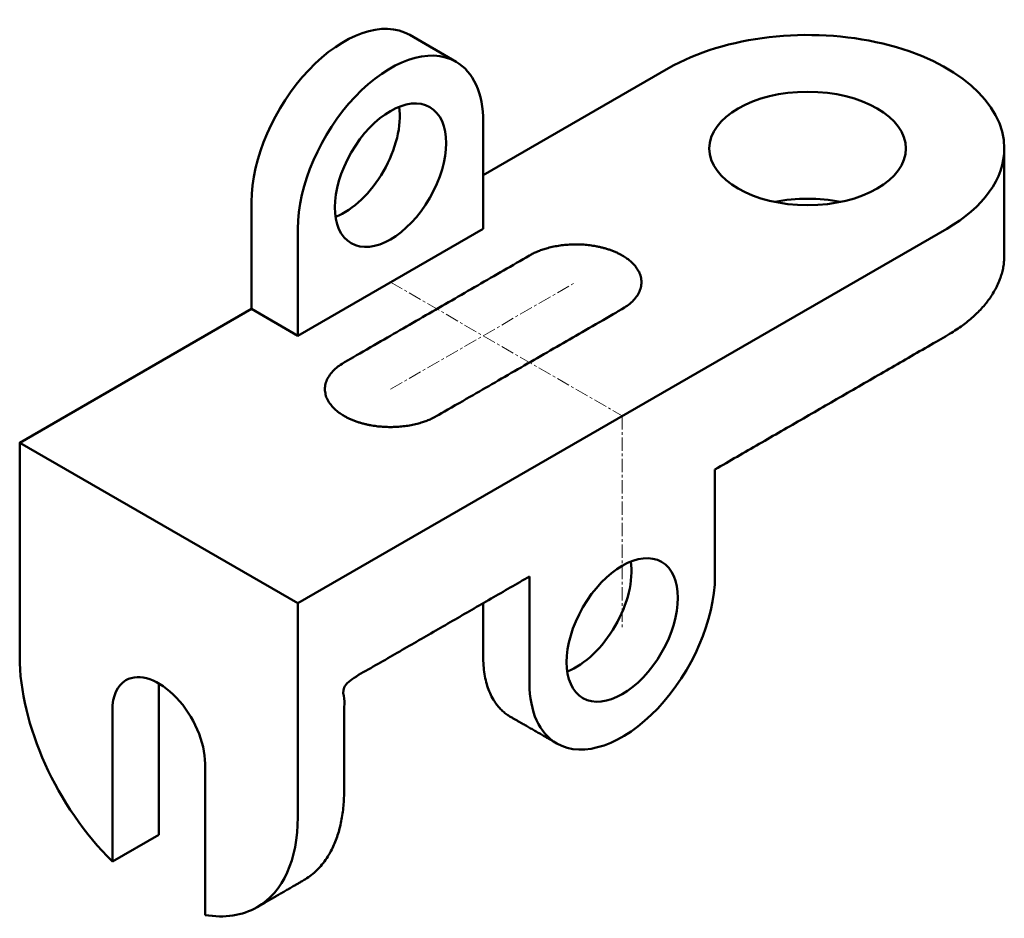
# Model space of a CAD drawing. Units: millimetres. Extents: x 1.1 to 93.1, y 18.3 to 102.2.
import ezdxf

# ---------------------------------------------------------------- set-up
doc = ezdxf.new("R2010")
doc.units = ezdxf.units.MM
doc.header["$MEASUREMENT"] = 0
doc.linetypes.add('CENTER', pattern=[2, 1.25, -0.25, 0.25, -0.25])
doc.layers.add('M-CNTR', color=4, linetype='CENTER', lineweight=18)
doc.layers.add('M-OUTL', color=7, linetype='Continuous', lineweight=50)

msp = doc.modelspace()

# ---------------------------------------------------------------- linework, layer by layer
at = {"layer": 'M-CNTR'}
msp.add_line((35.757, 67.712), (53.077, 77.712), dxfattribs=at)
msp.add_lwpolyline([(35.757, 77.712), (57.408, 65.212), (57.408, 55.212), (57.408, 45.212)], dxfattribs=at)
at = {"layer": 'M-OUTL'}
for p, q in [((37.551, 100.819), (41.881, 98.319)), ((44.417, 87.712), (61.738, 97.712)), ((44.417, 82.712), (44.417, 92.712)), ((22.767, 85.212), (22.767, 75.212)), ((27.097, 47.712), (87.719, 82.712)), ((27.097, 72.712), (44.417, 82.712)), ((27.097, 82.712), (27.097, 72.712)), ((27.097, 72.712), (22.767, 75.212)), ((1.116, 62.712), (27.097, 47.712)), ((66.068, 60.212), (66.068, 50.212)), ((48.747, 40.212), (48.747, 50.212)), ((27.097, 47.712), (27.097, 27.712)), ((14.106, 26.07), (14.106, 40.212)), ((9.776, 37.712), (9.776, 23.57)), ((18.437, 18.57), (18.437, 32.712)), ((14.106, 26.07), (9.776, 23.57))]:
    msp.add_line(p, q, dxfattribs=at)
msp.add_lwpolyline([(22.767, 75.212), (1.116, 62.712), (1.116, 42.712)], dxfattribs=at)
for centre, major_axis, start_param, end_param in [((31.427, 90.212), (-6.124, -10.607), 3.141593, 5.497787), ((74.728, 90.212), (18.371, 0), 0, 2.356194), ((35.757, 87.712), (-6.124, -10.607), 3.141593, 5.497787), ((35.757, 87.712), (-6.124, -10.607), 2.356194, 3.141593), ((31.427, 90.212), (3.674, 6.364), 3.77173, 5.653048), ((74.728, 90.212), (18.371, 0), 5.497787, 6.283185), ((74.728, 80.212), (-9.186, 0), 4.372552, 5.052226), ((53.077, 47.712), (-3.674, -6.364), 6.913323, 8.794641), ((57.408, 45.212), (6.124, 10.607), 3.141593, 5.497787), ((14.106, 35.212), (-9.186, 15.91), 0.785398, 2.016358), ((14.106, 35.212), (-3.062, 5.303), 0, 0.785398), ((14.106, 35.212), (-3.062, 5.303), 3.926991, 6.283185), ((57.408, 45.212), (6.124, 10.607), 2.356194, 3.141593), ((14.106, 35.212), (-9.186, 15.91), 3.141593, 3.926991), ((14.106, 35.212), (-9.186, 15.91), 2.696031, 3.141593)]:
    msp.add_ellipse(centre, major_axis=major_axis, ratio=0.57735, start_param=start_param, end_param=end_param, dxfattribs=at)
for centre, major_axis in [((35.757, 87.712), (-3.674, -6.364)), ((74.728, 90.212), (-9.186, 0)), ((57.408, 45.212), (-3.674, -6.364))]:
    msp.add_ellipse(centre, major_axis=major_axis, ratio=0.57735, dxfattribs=at)
for points, weights, knots in [([(66.068, 60.212), (76.893, 66.462), (87.719, 72.712), (93.099, 75.818), (93.099, 80.212), (93.099, 85.212), (93.099, 90.212)], [1, 1, 1, 0.923879532511, 1, 1, 1], [0, 0, 0, 1, 1, 1.785398, 1.785398, 2.785398, 2.785398, 2.785398]), ([(48.747, 80.212), (40.087, 75.212), (31.427, 70.212), (28.927, 68.768), (29.842, 66.797), (30.757, 64.825), (34.172, 64.297), (37.587, 63.768), (40.087, 65.212), (48.747, 70.212), (57.408, 75.212), (59.908, 76.655), (58.993, 78.627), (58.077, 80.598), (54.662, 81.127), (51.247, 81.655), (48.747, 80.212)], [1, 1, 1, 0.866025403784, 1, 0.866025403784, 1, 0.866025403784, 1, 1, 1, 0.866025403784, 1, 0.866025403784, 1, 0.866025403784, 1], [0, 0, 0, 1, 1, 2.047198, 2.047198, 3.094395, 3.094395, 4.141593, 4.141593, 5.141593, 5.141593, 6.18879, 6.18879, 7.235988, 7.235988, 8.283185, 8.283185, 8.283185]), ([(23.292, 19.302), (25.457, 20.552), (27.622, 21.802), (31.427, 23.998), (31.427, 30.212), (31.427, 35.212), (31.427, 40.212), (40.087, 45.212), (48.747, 50.212)], [1, 1, 1, 0.923879532511, 1, 1, 1, 1, 1], [0, 0, 0, 1, 1, 1.785398, 1.785398, 2.785398, 2.785398, 3.785398, 3.785398, 3.785398]), ([(44.417, 47.712), (44.417, 45.212), (44.417, 42.712), (44.417, 38.564), (46.96, 37.102), (49.014, 35.92), (51.068, 34.739)], [1, 1, 1, 0.92369523499, 1, 1, 1], [0, 0, 0, 1, 1, 1.786361, 1.786361, 2.786361, 2.786361, 2.786361])]:
    msp.add_rational_spline(points, weights, degree=2, knots=knots, dxfattribs=at)

doc.saveas('drawing.dxf')
